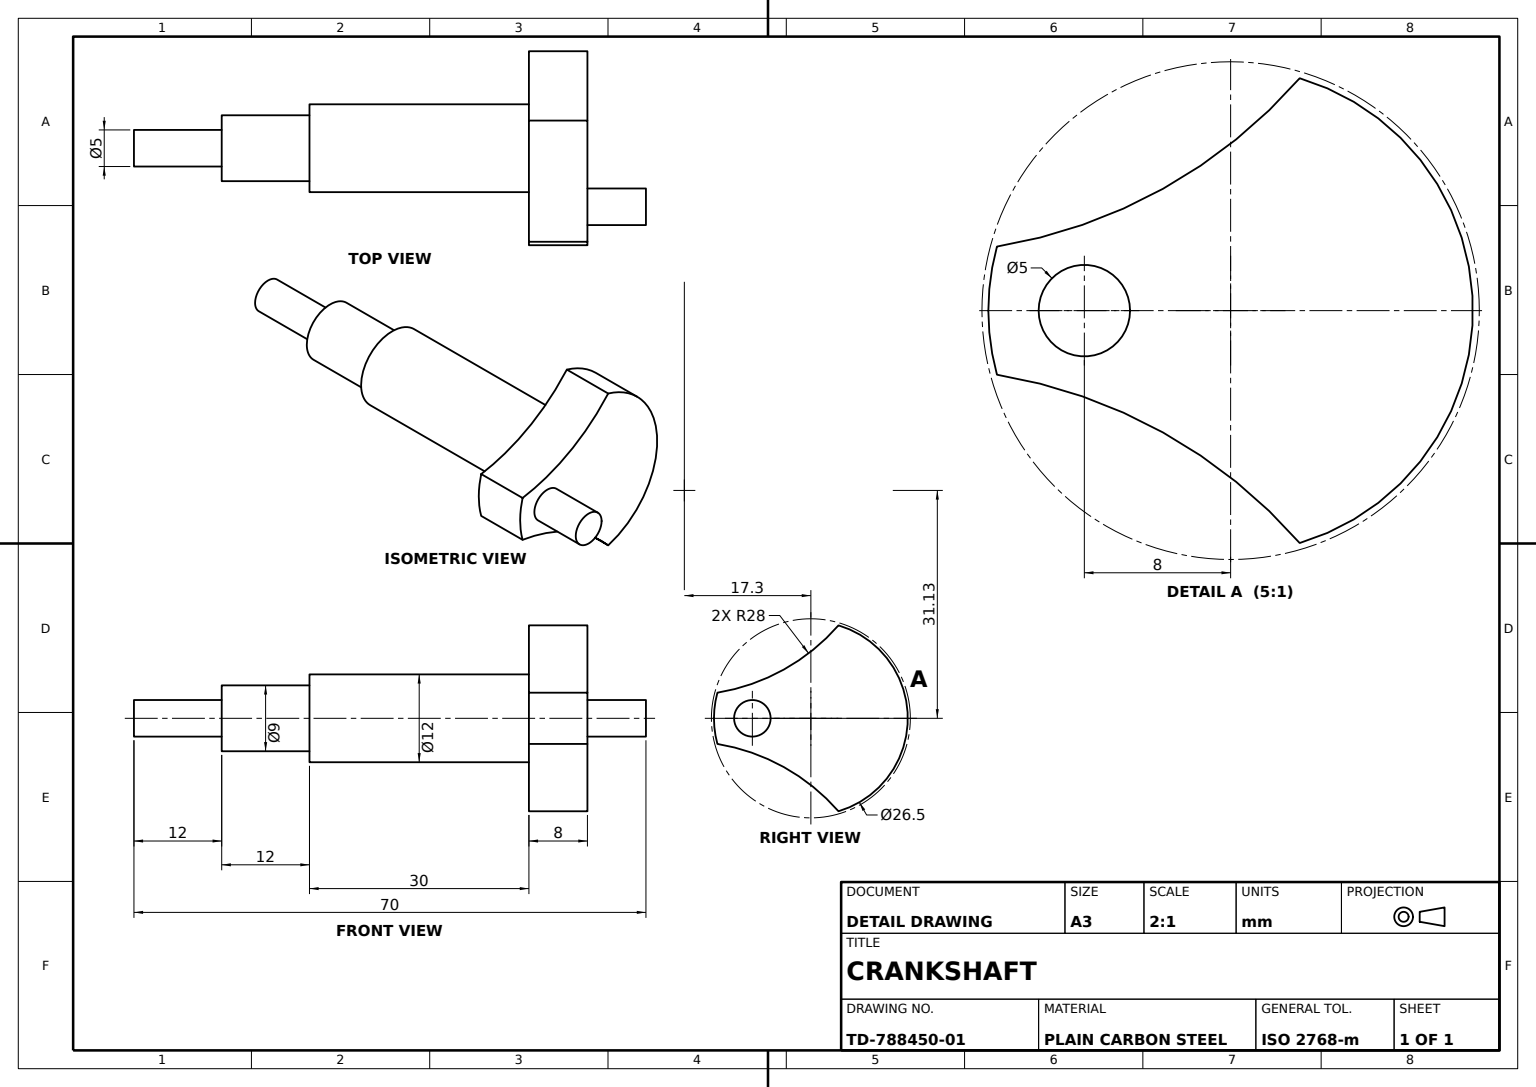
SolidWorks part; units mm, degrees
material "Plain Carbon Steel"
ref_plane "Front Plane" through (0, 0, 0) normal (0, 0, 1) x (1, 0, 0)
ref_plane "Top Plane" through (0, 0, 0) normal (0, 1, 0) x (1, 0, 0)
ref_plane "Right Plane" through (0, 0, 0) normal (1, 0, 0) x (0, 0, -1)
sketch "Main Journal Profile Ø12" plane through (0, 0, 0) normal (0, 0, 1) x (1, 0, 0)
  circle A0 centre (0, 0) radius 6
  dimension "D1" = 12
extrude "Main Journal Ø12" add sketch "Main Journal Profile Ø12" along normal blind 30
sketch "Step Journal Profile Ø9" plane through (0, 0, 30) normal (0, 0, 1) x (1, 0, 0)
  circle A0 centre (0, 0) radius 4.5
  dimension "D1" = 9
extrude "Step Journal Ø9" add sketch "Step Journal Profile Ø9" along normal blind 12
sketch "Shaft End Profile Ø5" plane through (0, 0, 42) normal (0, 0, 1) x (1, 0, 0)
  circle A0 centre (0, 0) radius 2.5
  dimension "D1" = 5
extrude "Shaft End Ø5" add sketch "Shaft End Profile Ø5" along normal blind 12
sketch "Crank Web Profile" plane through (0, 0, 0) normal (0, 0, -1) x (-1, 0, 0)
  line L0 (-16.7976, 0) -> (8.6866, 0) construction
  arc A0 (-12.7794, 3.5) -> (-12.7794, -3.5) centre (0, 0) ccw
  arc A1 (-12.7794, 3.5) -> (3.7778, 12.7) centre (-17.299, 31.1328) ccw
  arc A2 (-12.7794, -3.5) -> (3.7778, -12.7) centre (-17.299, -31.1328) cw
  arc A3 (3.7778, -12.7) -> (3.7778, 12.7) centre (0, 0) ccw
  circle A4 centre (0, 0) radius 6 construction
  dimension "D1" = 26.5
  dimension "D3" = 28
  dimension "D2" = 3.7778
  dimension "D4" = 12.7794
extrude "Crank Web" add sketch "Crank Web Profile" along normal blind 8
sketch "Crank Pin Profile" plane through (0, 0, -8) normal (0, 0, -1) x (-1, 0, 0)
  circle A0 centre (-8, 0) radius 2.5
  arc A1 (-12.7794, 3.5) -> (3.7778, 12.7) centre (-17.299, 31.1328) ccw construction
  dimension "D2" = 5
  dimension "D1" = 8
  dimension "D3" = 32.4919
extrude "Crank Pin" add sketch "Crank Pin Profile" along normal blind 8
